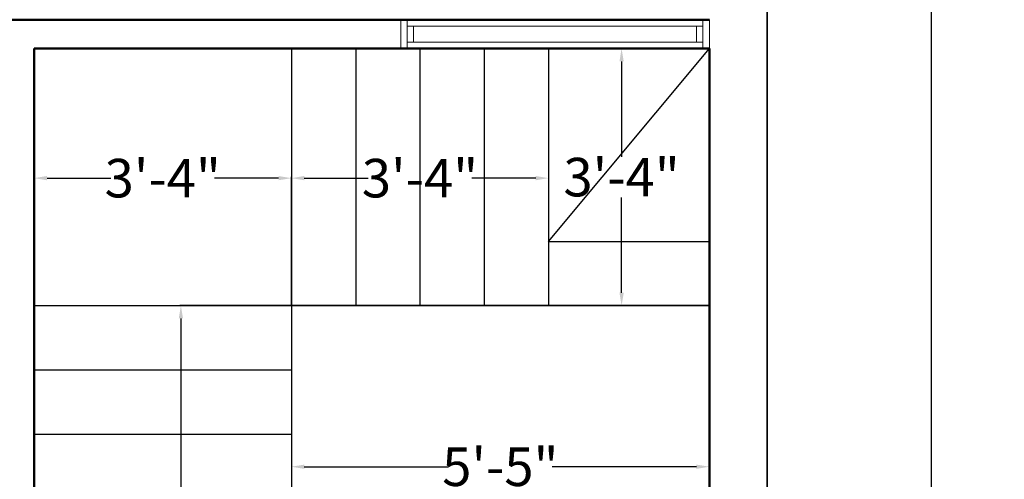
# Model space of a CAD drawing. Units: inches. Extents: x 134 to 568, y 15 to 554.
# Tile 5 of 7: x 415 to 568, y 164 to 235. Entities that reach past the tile are written whole.
import ezdxf

# ---------------------------------------------------------------- set-up
doc = ezdxf.new("R2010")
doc.units = ezdxf.units.IN
doc.header["$MEASUREMENT"] = 0
for name, color, linetype, lineweight in [('A-ANNO-DIMS', 2, 'Continuous', 18), ('A-FLOR-STRS', 3, 'Continuous', 25), ('A-GLAZ', 4, 'Continuous', 18), ('A-WALL', 7, 'Continuous', 50), ('C-PROP', 7, 'Continuous', 35)]:
    doc.layers.add(name, color=color, linetype=linetype, lineweight=lineweight)
doc.styles.get("Standard").update_dxf_attribs({"font": 'arial.ttf'})
doc.dimstyles.get("Standard").update_dxf_attribs({"dimtxt": 6, "dimasz": 2, "dimexe": 0.18, "dimexo": 0.0625, "dimgap": 0.09, "dimtad": 0, "dimtih": 1, "dimtoh": 1, "dimdec": 0, "dimzin": 0, "dimdsep": 46, "dimlunit": 4, "dimtxsty": 'Standard', "dimcen": 0.09, "dimadec": 0, "dimazin": 0, "dimtfac": 1, "dimtdec": 0, "dimtofl": 0, "dimtmove": 0, "dimatfit": 3, "dimfxl": 1, "dimtolj": 1, "dimtzin": 0, "dimarcsym": 0})

# ---------------------------------------------------------------- blocks, each defined once
blk = doc.blocks.new('*D2')
at = {"layer": 'A-ANNO-DIMS', "color": 0, "lineweight": -2, "transparency": 16777216}
for p, q in [((457.08, 190.52), (457.08, 165.33)), ((522.08, 190.52), (522.08, 165.33)), ((459.08, 165.51), (481.52, 165.51)), ((520.08, 165.51), (497.65, 165.51))]:
    blk.add_line(p, q, dxfattribs=at)
at = {"layer": 'A-ANNO-DIMS', "color": 0, "transparency": 16777216}
for points in [[(459.08, 165.84), (459.08, 165.18), (457.08, 165.51)], [(520.08, 165.84), (520.08, 165.18), (522.08, 165.51)]]:
    blk.add_solid(points, dxfattribs=at)
at = {"layer": 'Defpoints', "color": 0, "transparency": 16777216}
for p in [(457.08, 190.58), (522.08, 190.58), (522.08, 165.51)]:
    blk.add_point(p, dxfattribs=at)
at = {"layer": 'A-ANNO-DIMS', "color": 0, "transparency": 16777216, "insert": (489.58, 165.51), "char_height": 6, "attachment_point": 5}
blk.add_mtext('\\A1;5\'-5"', dxfattribs=at)
blk = doc.blocks.new('*D3')
at = {"layer": 'A-ANNO-DIMS', "color": 0, "lineweight": -2, "transparency": 16777216}
for p, q in [((417.08, 190.64), (417.08, 210.6)), ((419.08, 210.42), (429.02, 210.42)), ((455.08, 210.42), (445.15, 210.42)), ((457.08, 190.64), (457.08, 210.6))]:
    blk.add_line(p, q, dxfattribs=at)
at = {"layer": 'A-ANNO-DIMS', "color": 0, "transparency": 16777216}
for points in [[(419.08, 210.75), (419.08, 210.09), (417.08, 210.42)], [(455.08, 210.75), (455.08, 210.09), (457.08, 210.42)]]:
    blk.add_solid(points, dxfattribs=at)
at = {"layer": 'Defpoints', "color": 0, "transparency": 16777216}
for p in [(417.08, 210.42), (417.08, 190.58), (457.08, 190.58)]:
    blk.add_point(p, dxfattribs=at)
at = {"layer": 'A-ANNO-DIMS', "color": 0, "transparency": 16777216, "insert": (437.08, 210.42), "char_height": 6, "attachment_point": 5}
blk.add_mtext('\\A1;3\'-4"', dxfattribs=at)
blk = doc.blocks.new('*D4')
at = {"layer": 'A-ANNO-DIMS', "color": 0, "lineweight": -2, "transparency": 16777216}
for p, q in [((457.08, 230.52), (457.08, 210.24)), ((497.08, 230.52), (497.08, 210.24)), ((459.08, 210.42), (469.02, 210.42)), ((495.08, 210.42), (485.15, 210.42))]:
    blk.add_line(p, q, dxfattribs=at)
at = {"layer": 'A-ANNO-DIMS', "color": 0, "transparency": 16777216}
for points in [[(459.08, 210.75), (459.08, 210.09), (457.08, 210.42)], [(495.08, 210.75), (495.08, 210.09), (497.08, 210.42)]]:
    blk.add_solid(points, dxfattribs=at)
at = {"layer": 'Defpoints', "color": 0, "transparency": 16777216}
for p in [(457.08, 230.58), (497.08, 230.58), (497.08, 210.42)]:
    blk.add_point(p, dxfattribs=at)
at = {"layer": 'A-ANNO-DIMS', "color": 0, "transparency": 16777216, "insert": (477.08, 210.42), "char_height": 6, "attachment_point": 5}
blk.add_mtext('\\A1;3\'-4"', dxfattribs=at)
blk = doc.blocks.new('*D5')
at = {"layer": 'A-ANNO-DIMS', "color": 0, "lineweight": -2, "transparency": 16777216}
for p, q in [((522.02, 230.58), (508.25, 230.58)), ((508.43, 228.58), (508.43, 213.74)), ((508.43, 192.58), (508.43, 207.43)), ((522.02, 190.58), (508.25, 190.58))]:
    blk.add_line(p, q, dxfattribs=at)
at = {"layer": 'A-ANNO-DIMS', "color": 0, "transparency": 16777216}
for points in [[(508.1, 228.58), (508.77, 228.58), (508.43, 230.58)], [(508.1, 192.58), (508.77, 192.58), (508.43, 190.58)]]:
    blk.add_solid(points, dxfattribs=at)
at = {"layer": 'Defpoints', "color": 0, "transparency": 16777216}
for p in [(522.08, 230.58), (508.43, 190.58), (522.08, 190.58)]:
    blk.add_point(p, dxfattribs=at)
at = {"layer": 'A-ANNO-DIMS', "color": 0, "transparency": 16777216, "insert": (508.43, 210.58), "char_height": 6, "attachment_point": 5}
blk.add_mtext('\\A1;3\'-4"', dxfattribs=at)
blk = doc.blocks.new('*D6')
at = {"layer": 'A-ANNO-DIMS', "color": 0, "lineweight": -2, "transparency": 16777216}
for p, q in [((522.02, 190.58), (439.72, 190.58)), ((439.9, 188.58), (439.9, 120.68)), ((439.9, 46.58), (439.9, 114.48)), ((522.02, 44.58), (439.72, 44.58))]:
    blk.add_line(p, q, dxfattribs=at)
at = {"layer": 'A-ANNO-DIMS', "color": 0, "transparency": 16777216}
for points in [[(439.57, 188.58), (440.23, 188.58), (439.9, 190.58)], [(439.57, 46.58), (440.23, 46.58), (439.9, 44.58)]]:
    blk.add_solid(points, dxfattribs=at)
at = {"layer": 'Defpoints', "color": 0, "transparency": 16777216}
for p in [(439.9, 190.58), (522.08, 190.58), (522.08, 44.58)]:
    blk.add_point(p, dxfattribs=at)
at = {"layer": 'A-ANNO-DIMS', "color": 0, "transparency": 16777216, "insert": (439.9, 117.58), "char_height": 6, "attachment_point": 5}
blk.add_mtext('\\A1;12\'-2"', dxfattribs=at)
blk = doc.blocks.new('window 4.5')
for p, q in [((346.58, -32.94), (346.58, -28.44)), ((346.58, -28.44), (394.58, -28.44)), ((347.58, -32.94), (347.58, -28.44)), ((393.58, -28.44), (393.58, -32.94)), ((394.58, -28.44), (394.58, -32.94)), ((347.58, -29.44), (393.58, -29.44)), ((348.58, -31.94), (348.58, -29.44)), ((392.58, -29.44), (392.58, -31.94)), ((393.58, -31.94), (347.58, -31.94)), ((394.58, -32.94), (346.58, -32.94))]:
    blk.add_line(p, q)
blk = doc.blocks.new('*D60')
at = {"layer": 'A-ANNO-DIMS', "color": 0, "lineweight": -2, "transparency": 16777216}
for p, q in [((522.15, 515.58), (556.81, 515.58)), ((556.63, 513.58), (556.63, 283.24)), ((556.63, 46.58), (556.63, 276.93)), ((522.15, 44.58), (556.81, 44.58))]:
    blk.add_line(p, q, dxfattribs=at)
at = {"layer": 'A-ANNO-DIMS', "color": 0, "transparency": 16777216}
for points in [[(556.3, 513.58), (556.97, 513.58), (556.63, 515.58)], [(556.3, 46.58), (556.97, 46.58), (556.63, 44.58)]]:
    blk.add_solid(points, dxfattribs=at)
at = {"layer": 'Defpoints', "color": 0, "transparency": 16777216}
for p in [(522.08, 515.58), (556.63, 515.58), (522.08, 44.58)]:
    blk.add_point(p, dxfattribs=at)
at = {"layer": 'A-ANNO-DIMS', "color": 0, "transparency": 16777216, "insert": (556.63, 280.08), "char_height": 6, "attachment_point": 5}
blk.add_mtext('\\A1;39\'-3"', dxfattribs=at)

msp = doc.modelspace()

# ---------------------------------------------------------------- linework, layer by layer
at = {"layer": 'A-FLOR-STRS'}
for p, q in [((457.08, 230.58), (457.08, 110.58)), ((467.08, 230.58), (467.08, 190.58)), ((477.08, 230.58), (477.08, 190.58)), ((487.08, 230.58), (487.08, 190.58)), ((497.08, 230.58), (497.08, 190.58)), ((497.08, 200.58), (522.08, 230.58)), ((497.08, 200.58), (522.08, 200.58)), ((417.08, 190.58), (522.08, 190.58)), ((417.08, 180.58), (457.08, 180.58)), ((417.08, 170.58), (457.08, 170.58))]:
    msp.add_line(p, q, dxfattribs=at)
at = {"layer": 'A-WALL'}
for p, q in [((402.08, 235.08), (522.08, 235.08)), ((417.08, 230.58), (417.08, 110.58)), ((417.08, 230.58), (522.08, 230.58)), ((522.08, 44.58), (522.08, 230.58))]:
    msp.add_line(p, q, dxfattribs=at)
at = {"layer": 'C-PROP'}
msp.add_line((531.08, 44.58), (531.08, 524.58), dxfattribs=at)

# ---------------------------------------------------------------- block references
at = {"layer": 'A-GLAZ'}
msp.add_blockref('window 4.5', (127.5, 263.52), dxfattribs=at)

# ---------------------------------------------------------------- dimensions: what is measured, and where the dimension line sits
at = {"layer": 'A-ANNO-DIMS'}
for base, p1, p2, override, picture, middle in [((556.63, 515.58), (522.08, 44.58), (522.08, 515.58), {"dimdec": 1, "dimlfac": 1, "dimrnd": 0, "dimzin": 1, "dimdsep": 46, "dimlunit": 4, "dimfrac": 2}, '*D60', (556.63, 280.08)), ((508.43, 190.58), (522.08, 230.58), (522.08, 190.58), {"dimclrd": 0, "dimclre": 0, "dimclrt": 0}, '*D5', (508.43, 210.58)), ((439.9, 190.58), (522.08, 44.58), (522.08, 190.58), {"dimclrd": 0, "dimclre": 0, "dimclrt": 0}, '*D6', (439.9, 117.58))]:
    dim = msp.add_linear_dim(base=base, p1=p1, p2=p2, angle=90, dimstyle='Standard', override=override, dxfattribs=at)
    dim.commit()
    dim.dimension.update_dxf_attribs({"geometry": picture, "text_midpoint": middle})
for base, p1, p2, picture, middle in [((497.08, 210.42), (457.08, 230.58), (497.08, 230.58), '*D4', (477.08, 210.42)), ((417.08, 210.42), (457.08, 190.58), (417.08, 190.58), '*D3', (437.08, 210.42)), ((522.08, 165.51), (457.08, 190.58), (522.08, 190.58), '*D2', (489.58, 165.51))]:
    dim = msp.add_linear_dim(base=base, p1=p1, p2=p2, dimstyle='Standard', override={"dimclrd": 0, "dimclre": 0, "dimclrt": 0}, dxfattribs=at)
    dim.commit()
    dim.dimension.update_dxf_attribs({"geometry": picture, "text_midpoint": middle})

doc.saveas('drawing.dxf')
